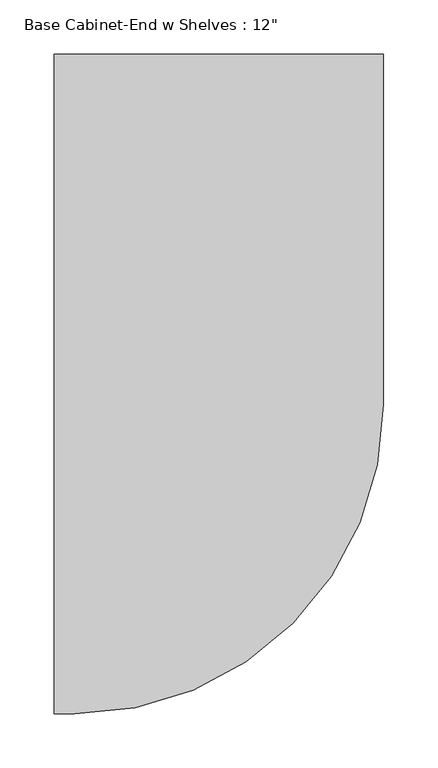
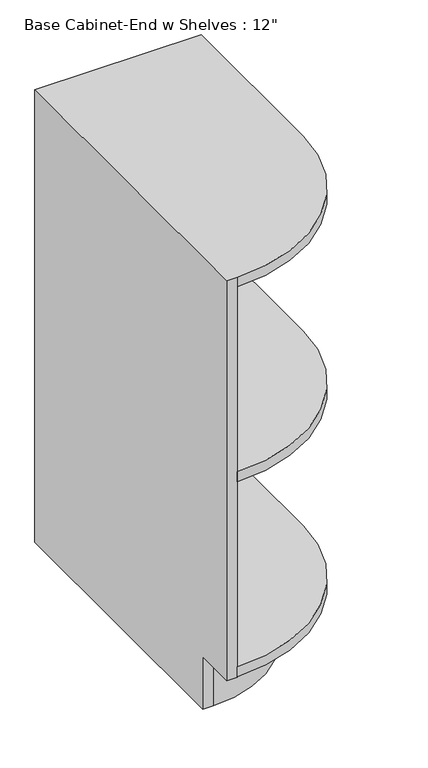
"""IFC4 building model written with IfcOpenShell, lengths in millimetres: furniture geometry."""

from ifc_helpers import new_model, si_unit, point, frame, frame_2d, origin, place, context, project, spatial, polyline, circle_curve, trimmed, segment, composite_curve, outline, extrude, source, transform, mapped, element, save
from ifc_brep_helpers import plane_surface, cylinder_surface, advanced_brep


def furniture_4ce329b2(model_context):
    return source(origin(), model_context, "Body", "SolidModel", [
        extrude(outline(composite_curve([segment(polyline([(304.8, -12.7), (304.8, -323.85)]), True, "CONTINUOUS"), segment(trimmed(circle_curve(frame_2d((19.05, -323.85)), 285.75), [point((304.8, -323.85))], [point((19.05, -609.6))], False, "CARTESIAN"), True, "CONTINUOUS"), segment(polyline([(19.05, -609.6), (19.05, -12.7), (304.8, -12.7)]), True, "CONTINUOUS")], self_intersect=False)), frame((0.0, 0.0, 480.615625), z_axis=(0.0, 0.0, 1.0), x_axis=(1.0, 0.0, 0.0)), (0.0, 0.0, 1.0), 19.05),
        advanced_brep(
        [(228.6, 0.0, 0.0), (228.6, -323.8500002, 0.0), (19.0500002, -533.4, 0.0), (0.0, -533.4, 0.0), (0.0, 0.0, 0.0), (0.0, 0.0, 877.490625), (304.8, 0.0, 877.490625), (304.8, 0.0, 101.6), (228.6, 0.0, 101.6), (0.0, -533.4, 101.6), (0.0, -609.6, 101.6), (0.0, -609.6, 877.490625), (19.0500002, -533.4, 101.6), (228.6, -323.8500002, 102.790625), (19.0500002, -533.4, 102.790625), (228.6, -12.7, 101.6), (228.6, -12.7, 102.790625), (19.05, -609.5999998, 121.840625), (304.8, -323.8499999, 121.840625), (304.8, -12.7, 121.840625), (19.05, -12.7, 121.840625), (304.8, -12.7, 102.790625), (304.8, -323.8499999, 102.790625), (19.05, -609.5999998, 102.790625), (304.8, -12.7, 101.6), (304.8, -323.85, 877.490625), (304.8, -323.85, 858.440625), (304.8, -12.7, 858.440625), (19.05, -609.6, 877.490625), (19.05, -609.6, 101.6), (19.05, -609.6, 858.440625), (19.05, -12.7, 858.440625)],
        [
            (0, 1),
            (1, 2, circle_curve(frame((19.0500002, -323.8500002, 0.0), z_axis=(0.0, 0.0, -1.0), x_axis=(1.0, 0.0, 0.0)), 209.5499998)),
            (2, 3),
            (3, 4),
            (4, 0),
            (4, 5),
            (5, 6),
            (6, 7),
            (7, 8),
            (8, 0),
            (3, 9),
            (9, 10),
            (10, 11),
            (11, 5),
            (2, 12),
            (12, 9),
            (1, 13),
            (13, 14, circle_curve(frame((19.0500002, -323.8500002, 102.790625), z_axis=(0.0, 0.0, -1.0), x_axis=(1.0, 0.0, 0.0)), 209.5499998)),
            (14, 12),
            (8, 15),
            (15, 16),
            (16, 13),
            (17, 18, circle_curve(frame((19.05, -323.8499999, 121.840625), z_axis=(0.0, 0.0, 1.0), x_axis=(1.0, 0.0, 0.0)), 285.75)),
            (18, 19),
            (19, 20),
            (20, 17),
            (21, 22),
            (22, 23, circle_curve(frame((19.05, -323.8499999, 102.790625), z_axis=(0.0, 0.0, -1.0), x_axis=(1.0, 0.0, 0.0)), 285.75)),
            (23, 14),
            (16, 21),
            (17, 23),
            (22, 18),
            (21, 24),
            (24, 7),
            (6, 25),
            (25, 26),
            (26, 27),
            (27, 19),
            (11, 28),
            (28, 25, circle_curve(frame((19.05, -323.85, 877.490625), z_axis=(0.0, 0.0, 1.0), x_axis=(1.0, 0.0, 0.0)), 285.75)),
            (29, 10),
            (12, 29),
            (29, 23),
            (17, 30),
            (30, 28),
            (20, 31),
            (31, 30),
            (24, 15),
            (27, 31),
            (26, 30, circle_curve(frame((19.05, -323.85, 858.440625), z_axis=(0.0, 0.0, -1.0), x_axis=(1.0, 0.0, 0.0)), 285.75)),
        ],
        [
            plane_surface(frame((0.0, 0.0, 0.0), z_axis=(0.0, 0.0, -1.0), x_axis=(1.0, 0.0, 0.0))),
            plane_surface(frame((228.6, 0.0, 102.790625), z_axis=(0.0, 1.0, 0.0), x_axis=(0.0, 0.0, -1.0))),
            plane_surface(frame((0.0, 0.0, 102.790625), z_axis=(-1.0, 0.0, 0.0), x_axis=(0.0, 0.0, -1.0))),
            plane_surface(frame((0.0, -533.4, 102.790625), z_axis=(0.0, -1.0, 0.0), x_axis=(0.0, 0.0, -1.0))),
            cylinder_surface(frame((19.0500002, -323.8500002, 0.0), z_axis=(0.0, 0.0, 1.0), x_axis=(1.0, 0.0, 0.0)), 209.5499998),
            plane_surface(frame((228.6, -323.8500002, 102.790625), z_axis=(1.0, 0.0, 0.0), x_axis=(0.0, 0.0, -1.0))),
            plane_surface(frame((304.8, -12.7, 121.840625), z_axis=(0.0, 0.0, 1.0), x_axis=(-1.0, 0.0, 0.0))),
            plane_surface(frame((304.8, -12.7, 102.790625), z_axis=(0.0, 0.0, -1.0), x_axis=(1.0, 0.0, 0.0))),
            cylinder_surface(frame((19.05, -323.8499999, 102.790625), z_axis=(0.0, 0.0, 1.0), x_axis=(1.0, 0.0, 0.0)), 285.75),
            plane_surface(frame((304.8, -323.8499999, 121.840625), z_axis=(1.0, 0.0, 0.0), x_axis=(0.0, 0.0, -1.0))),
            plane_surface(frame((0.0, -431.0601378, 877.490625), z_axis=(0.0, 0.0, 1.0), x_axis=(0.0, -1.0, 0.0))),
            plane_surface(frame((0.0, -431.0601378, 101.6), z_axis=(0.0, 0.0, -1.0), x_axis=(0.0, 1.0, 0.0))),
            plane_surface(frame((0.0, -609.6, 877.490625), z_axis=(0.0, -1.0, 0.0), x_axis=(0.0, 0.0, -1.0))),
            plane_surface(frame((19.05, -609.6, 877.490625), z_axis=(1.0, 0.0, 0.0), x_axis=(0.0, 0.0, -1.0))),
            plane_surface(frame((19.05, 0.0, 101.6), z_axis=(0.0, 0.0, -1.0), x_axis=(1.0, 0.0, 0.0))),
            plane_surface(frame((19.05, -12.7, 877.490625), z_axis=(0.0, -1.0, 0.0), x_axis=(0.0, 0.0, -1.0))),
            plane_surface(frame((19.05, -12.7, 858.440625), z_axis=(0.0, 0.0, -1.0), x_axis=(0.0, 1.0, 0.0))),
            cylinder_surface(frame((19.05, -323.85, 858.440625), z_axis=(0.0, 0.0, 1.0), x_axis=(1.0, 0.0, 0.0)), 285.75),
        ],
        [
            (0, [[1, 2, 3, 4, 5]]),
            (1, [[-5, 6, 7, 8, 9, 10]]),
            (2, [[-4, 11, 12, 13, 14, -6]]),
            (3, [[-3, 15, 16, -11]]),
            (4, [[-2, 17, 18, 19, -15]]),
            (5, [[-1, -10, 20, 21, 22, -17]]),
            (6, [[23, 24, 25, 26]]),
            (7, [[27, 28, 29, -18, -22, 30]]),
            (8, [[-23, 31, -28, 32]]),
            (9, [[-24, -32, -27, 33, 34, -8, 35, 36, 37, 38]]),
            (10, [[-14, 39, 40, -35, -7]]),
            (11, [[41, -12, -16, 42]]),
            (12, [[-39, -13, -41, 43, -31, 44, 45]]),
            (13, [[-26, 46, 47, -44]]),
            (13, [[-42, -19, -29, -43]]),
            (14, [[-34, 48, -20, -9]]),
            (15, [[-25, -38, 49, -46]]),
            (15, [[-33, -30, -21, -48]]),
            (16, [[-37, 50, -47, -49]]),
            (17, [[-40, -45, -50, -36]]),
        ],
    ),
    ])


if __name__ == "__main__":
    model = new_model("IFC4")
    model_context = context("Model", 3, world=origin())
    ifc_project = project(units=[si_unit("LENGTHUNIT", "METRE", prefix="MILLI")], contexts=[model_context])
    site = spatial("IfcSite", under=ifc_project)
    building = spatial("IfcBuilding", under=site)
    placement = place(None, origin())
    furniture_shape = furniture_4ce329b2(model_context)
    element("IfcFurniture", 1, ObjectType="Base Cabinet-End w Shelves : 12\"", at=placement, inside=building, context=model_context, shape_type="MappedRepresentation", body=[
        mapped(furniture_shape, transform((0.0, 0.0, 0.0), x_axis=(1.0, 0.0, 0.0), y_axis=(0.0, 1.0, 0.0), z_axis=(0.0, 0.0, 1.0))),
    ])
    save(model, "model.ifc")

# Revit data of these elements
# Type "Base Cabinet-End w Shelves : 12\""
#   Assembly Code = "C1030410"
#   Width = 1' - 0"
#   Toe Kick Depth = 0' - 3"
#   Height = 2' - 10 1/2"
#   Depth = 2' - 0"
#   Cabinet Material = Cabinets
#   Default Elevation = 0
# Element 1 (IfcFurniture, "Base Cabinet-End w Shelves : 12\"")
#   Materials on its faces: "Cabinets"
# Materials
#   "Cabinets": colour RGB 249 249 249, transparency 0
